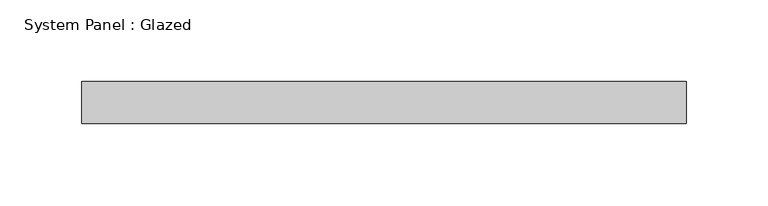
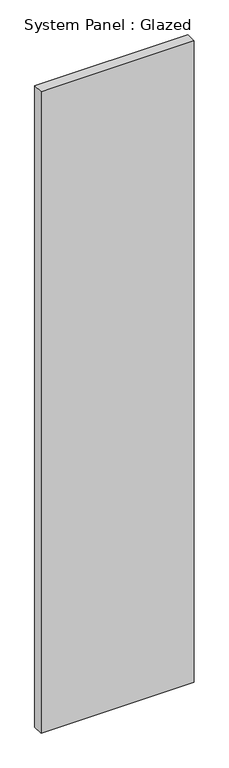
"""IFC4 building model written with IfcOpenShell, lengths in millimetres: plate geometry, System Panel : Glazed."""

from ifc_helpers import new_model, si_unit, origin, origin_with_axes, place, context, project, spatial, polyline, outline, extrude, source, transform, mapped, element, save


def system_panel_glazed_8729007e(model_context):
    return source(origin(), model_context, "Body", "SweptSolid", [
        extrude(outline(polyline([(184.15, 19.05), (-184.15, 19.05), (-184.15, 44.45), (184.15, 44.45), (184.15, 19.05)])), origin_with_axes(), (0.0, 0.0, 1.0), 1630.093674),
    ])


if __name__ == "__main__":
    model = new_model("IFC4")
    model_context = context("Model", 3, world=origin())
    ifc_project = project(units=[si_unit("LENGTHUNIT", "METRE", prefix="MILLI")], contexts=[model_context])
    site = spatial("IfcSite", under=ifc_project)
    building = spatial("IfcBuilding", under=site)
    placement = place(None, origin())
    system_panel_glazed_shape = system_panel_glazed_8729007e(model_context)
    element("IfcPlate", 1, ObjectType="System Panel : Glazed", at=placement, inside=building, context=model_context, shape_type="MappedRepresentation", body=[
        mapped(system_panel_glazed_shape, transform((0.0, 0.0, 0.0), x_axis=(1.0, 0.0, 0.0), y_axis=(0.0, 1.0, 0.0), z_axis=(0.0, 0.0, 1.0))),
    ])
    save(model, "model.ifc")

# Revit data of these elements
# Type "System Panel : Glazed"
#   Construction Type Id = "GSP4R"
#   Analytic Construction = "1/8 in Pilkington single glazing"
#   Visual Light Transmittance = 0.9
#   Solar Heat Gain Coefficient = 0.86
#   Heat Transfer Coefficient (U) = 1.18115 BTU/(h·ft²·°F)
#   Define Thermal Properties by = 1
# Element 1 (IfcPlate, "System Panel : Glazed")
#   Materials on its faces: "Glass"
# Materials
#   "Glass": class "Glass", colour RGB 0 128 192, transparency 0.75, Description = "Soda Lime Glass", Cost = 0
